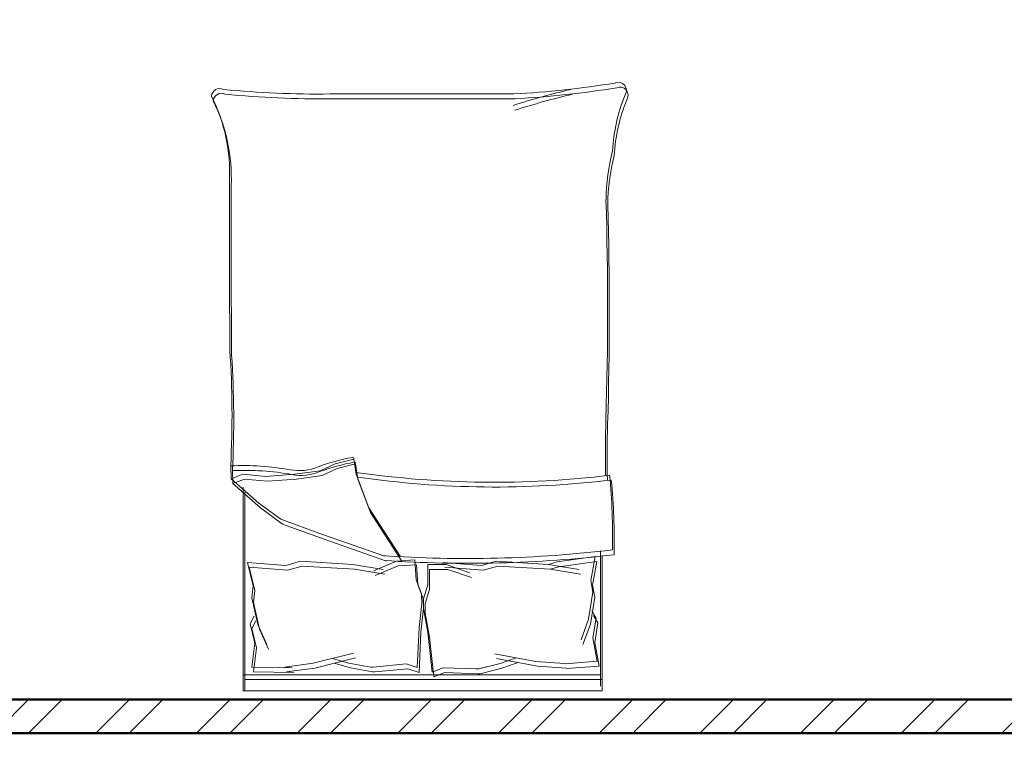
# Model space of a CAD drawing. Units: inches. Extents: x 963 to 2075, y 289 to 2657.
# Tile 15 of 98: x 1179 to 1310, y 1818 to 1917. Entities that reach past the tile are written whole.
import ezdxf

# ---------------------------------------------------------------- set-up
doc = ezdxf.new("R2010")
doc.units = ezdxf.units.IN
for name, color, linetype, lineweight in [('A-FURN', 8, 'Continuous', 18), ('A-WALL', 7, 'Continuous', 50), ('A-WALL-PATT', 8, 'Continuous', 13)]:
    doc.layers.add(name, color=color, linetype=linetype, lineweight=lineweight)

# ---------------------------------------------------------------- blocks, each defined once
blk = doc.blocks.new('BED-DOUBLE')
for p, q in [((1236.12, 2450.52), (1254.23, 2450.52)), ((1236.12, 2450.52), (1254.23, 2450.52)), ((1236.76, 2450.75), (1254.87, 2450.75)), ((1236.76, 2450.75), (1254.87, 2450.75)), ((1251.56, 2450.33), (1248.37, 2449.75)), ((1251.56, 2450.33), (1248.37, 2449.75)), ((1251.53, 2450.32), (1251.86, 2446.04)), ((1251.53, 2450.32), (1251.86, 2446.04)), ((1252.7, 2450.52), (1252.7, 2402.73)), ((1252.7, 2450.52), (1252.7, 2402.73)), ((1253.34, 2450.75), (1253.34, 2402.96)), ((1253.34, 2450.75), (1253.34, 2402.96)), ((1254.87, 2450.75), (1254.87, 2402.73)), ((1237.61, 2444.71), (1236.89, 2449.81)), ((1236.89, 2449.81), (1240.07, 2449.23)), ((1237.61, 2444.71), (1236.89, 2449.81)), ((1236.89, 2449.81), (1240.07, 2449.23)), ((1238.25, 2444.94), (1237.53, 2450.04)), ((1237.53, 2450.04), (1240.71, 2449.46)), ((1238.25, 2444.94), (1237.53, 2450.04)), ((1237.53, 2450.04), (1240.71, 2449.46)), ((1240.07, 2449.23), (1241.66, 2449.52)), ((1240.07, 2449.23), (1241.66, 2449.52)), ((1240.71, 2449.46), (1242.3, 2449.75)), ((1240.71, 2449.46), (1242.3, 2449.75)), ((1241.66, 2449.52), (1245.28, 2448.94)), ((1241.66, 2449.52), (1245.28, 2448.94)), ((1242.3, 2449.75), (1245.92, 2449.17)), ((1242.3, 2449.75), (1245.92, 2449.17)), ((1245.13, 2449.96), (1244.12, 2449.38)), ((1245.13, 2449.96), (1244.12, 2449.38)), ((1245.77, 2450.18), (1244.76, 2449.61)), ((1245.77, 2450.18), (1244.76, 2449.61)), ((1247.74, 2449.52), (1245.13, 2449.96)), ((1247.74, 2449.52), (1245.13, 2449.96)), ((1245.28, 2448.94), (1248.02, 2447.93)), ((1245.28, 2448.94), (1248.02, 2447.93)), ((1248.37, 2449.75), (1245.77, 2450.18)), ((1248.37, 2449.75), (1245.77, 2450.18)), ((1245.92, 2449.17), (1248.66, 2448.16)), ((1245.92, 2449.17), (1248.66, 2448.16)), ((1250.92, 2450.1), (1247.74, 2449.52)), ((1250.92, 2450.1), (1247.74, 2449.52)), ((1250.89, 2450.1), (1251.22, 2445.82)), ((1250.89, 2450.1), (1251.22, 2445.82)), ((1238.6, 2447.61), (1237.94, 2443.58)), ((1238.6, 2447.61), (1237.94, 2443.58)), ((1239.24, 2447.84), (1238.58, 2443.81)), ((1239.24, 2447.84), (1238.58, 2443.81)), ((1251.21, 2445.71), (1250.92, 2441.89)), ((1251.21, 2445.71), (1250.92, 2441.89)), ((1251.22, 2445.82), (1251.21, 2445.71)), ((1251.22, 2445.82), (1251.21, 2445.71)), ((1251.84, 2445.94), (1251.56, 2442.11)), ((1251.84, 2445.94), (1251.56, 2442.11)), ((1251.86, 2446.04), (1251.84, 2445.94)), ((1251.86, 2446.04), (1251.84, 2445.94)), ((1237.94, 2443.58), (1237.61, 2444.71)), ((1237.94, 2443.58), (1237.61, 2444.71)), ((1238.58, 2443.81), (1238.15, 2436.8)), ((1238.58, 2443.81), (1238.15, 2436.8)), ((1238.58, 2443.81), (1238.25, 2444.94)), ((1238.58, 2443.81), (1238.25, 2444.94)), ((1237.94, 2443.58), (1237.51, 2436.57)), ((1237.94, 2443.58), (1237.51, 2436.57)), ((1250.92, 2441.89), (1249.9, 2436.39)), ((1250.92, 2441.89), (1249.9, 2436.39)), ((1251.56, 2442.11), (1250.54, 2436.62)), ((1251.56, 2442.11), (1250.54, 2436.62)), ((1174.99, 2438.93), (1174.99, 2414.32)), ((1174.99, 2438.93), (1174.99, 2414.32)), ((1175.63, 2439.16), (1175.63, 2414.55)), ((1175.63, 2439.16), (1175.63, 2414.55)), ((1250.48, 2439.14), (1251.21, 2437.12)), ((1250.48, 2439.14), (1251.21, 2437.12)), ((1251.12, 2439.37), (1251.84, 2437.34)), ((1251.12, 2439.37), (1251.84, 2437.34)), ((1251.21, 2437.12), (1251.93, 2434.22)), ((1251.21, 2437.12), (1251.93, 2434.23)), ((1251.84, 2437.34), (1252.57, 2434.45)), ((1251.84, 2437.34), (1252.57, 2434.45)), ((1237.51, 2436.57), (1238.06, 2434.61)), ((1237.51, 2436.57), (1238.06, 2434.61)), ((1238.15, 2436.8), (1238.7, 2434.84)), ((1238.15, 2436.8), (1238.7, 2434.84)), ((1238.06, 2434.61), (1237.66, 2429.48)), ((1238.06, 2434.61), (1237.66, 2429.48)), ((1238.7, 2434.84), (1238.3, 2429.71)), ((1238.7, 2434.84), (1238.3, 2429.71)), ((1252.57, 2434.45), (1252.57, 2434.13)), ((1252.57, 2434.45), (1252.57, 2434.13)), ((1238.61, 2430.12), (1239.7, 2433.26)), ((1238.61, 2430.12), (1239.7, 2433.26)), ((1251.93, 2433.9), (1251.78, 2429.46)), ((1251.93, 2433.9), (1251.78, 2429.46)), ((1251.93, 2434.23), (1251.93, 2433.9)), ((1251.93, 2434.22), (1251.93, 2433.9)), ((1252.57, 2434.13), (1252.42, 2429.69)), ((1252.57, 2434.13), (1252.42, 2429.69)), ((1237.97, 2429.89), (1239.06, 2433.04)), ((1237.97, 2429.89), (1239.06, 2433.04)), ((1237.97, 2427.43), (1237.97, 2429.89)), ((1237.97, 2427.43), (1237.97, 2429.89)), ((1238.61, 2427.66), (1238.61, 2430.12)), ((1238.61, 2427.66), (1238.61, 2430.12)), ((1251.78, 2429.46), (1252.36, 2428.01)), ((1251.78, 2429.46), (1252.36, 2428.01)), ((1252.42, 2429.69), (1253, 2428.24)), ((1252.42, 2429.69), (1253, 2428.24)), ((1252.36, 2428.01), (1247.01, 2427.43)), ((1252.36, 2428.01), (1247.01, 2427.43)), ((1253, 2428.24), (1247.65, 2427.66)), ((1253, 2428.24), (1247.65, 2427.66)), ((1240.65, 2427.43), (1237.97, 2427.43)), ((1240.65, 2427.43), (1237.97, 2427.43)), ((1241.29, 2427.66), (1238.61, 2427.66)), ((1241.29, 2427.66), (1238.61, 2427.66)), ((1241.86, 2426.56), (1240.02, 2425.86)), ((1241.86, 2426.56), (1240.02, 2425.86)), ((1242.53, 2426.86), (1240.65, 2427.43)), ((1242.53, 2426.86), (1240.65, 2427.43)), ((1242.49, 2426.79), (1240.66, 2426.09)), ((1242.49, 2426.79), (1240.66, 2426.09)), ((1243.17, 2427.08), (1241.29, 2427.66)), ((1243.17, 2427.08), (1241.29, 2427.66)), ((1243.15, 2426.64), (1241.86, 2426.56)), ((1243.15, 2426.64), (1241.86, 2426.56)), ((1243.79, 2426.87), (1242.49, 2426.79)), ((1243.79, 2426.87), (1242.49, 2426.79)), ((1243.83, 2426.86), (1242.53, 2426.86)), ((1243.83, 2426.86), (1242.53, 2426.86)), ((1246.37, 2426.26), (1243.15, 2426.64)), ((1246.37, 2426.26), (1243.15, 2426.64)), ((1244.47, 2427.08), (1243.17, 2427.08)), ((1244.47, 2427.08), (1243.17, 2427.08)), ((1247, 2426.49), (1243.79, 2426.87)), ((1247, 2426.49), (1243.79, 2426.87)), ((1247.01, 2427.43), (1243.83, 2426.86)), ((1247.01, 2427.43), (1243.83, 2426.86)), ((1247.65, 2427.66), (1244.47, 2427.08)), ((1247.65, 2427.66), (1244.47, 2427.08)), ((1240.02, 2425.86), (1237.34, 2425.7)), ((1240.02, 2425.86), (1237.34, 2425.7)), ((1237.34, 2425.7), (1237.49, 2423.24)), ((1237.34, 2425.7), (1237.49, 2423.24)), ((1240.66, 2426.09), (1237.98, 2425.93)), ((1240.66, 2426.09), (1237.98, 2425.93)), ((1237.98, 2425.93), (1238.13, 2423.47)), ((1237.98, 2425.93), (1238.13, 2423.47)), ((1251.74, 2426.02), (1246.37, 2426.26)), ((1251.74, 2426.02), (1246.37, 2426.26)), ((1252.38, 2426.25), (1247, 2426.49)), ((1252.38, 2426.25), (1247, 2426.49)), ((1251.25, 2424.54), (1251.74, 2426.02)), ((1251.25, 2424.54), (1251.74, 2426.02)), ((1251.89, 2424.77), (1252.38, 2426.25)), ((1251.89, 2424.77), (1252.38, 2426.25)), ((1237.49, 2423.96), (1231, 2419.77)), ((1237.49, 2423.96), (1231, 2419.77)), ((1251.68, 2420.11), (1251.25, 2424.54)), ((1251.68, 2420.11), (1251.25, 2424.54)), ((1252.31, 2420.34), (1251.89, 2424.77)), ((1252.31, 2420.34), (1251.89, 2424.77)), ((1236.85, 2423.74), (1230.36, 2419.55)), ((1236.85, 2423.74), (1230.36, 2419.55)), ((1237.49, 2423.24), (1238.78, 2420.17)), ((1237.49, 2423.24), (1238.78, 2420.17)), ((1238.13, 2423.47), (1239.42, 2420.4)), ((1238.13, 2423.47), (1239.42, 2420.4)), ((1233.92, 2413.35), (1236.85, 2421.69)), ((1233.92, 2413.35), (1236.85, 2421.69)), ((1234.56, 2413.58), (1237.49, 2421.92)), ((1234.56, 2413.58), (1237.49, 2421.92)), ((1238.6, 2421.43), (1237.94, 2417.4)), ((1238.6, 2421.43), (1237.94, 2417.4)), ((1239.24, 2421.66), (1238.58, 2417.63)), ((1239.24, 2421.66), (1238.58, 2417.63)), ((1251.7, 2419.79), (1251.68, 2420.11)), ((1251.7, 2419.79), (1251.68, 2420.11)), ((1251.79, 2417.09), (1252.33, 2420.02)), ((1251.79, 2417.09), (1252.33, 2420.02)), ((1252.33, 2420.02), (1252.31, 2420.34)), ((1252.33, 2420.02), (1252.31, 2420.34)), ((1230.36, 2419.55), (1225.87, 2417.84)), ((1230.36, 2419.55), (1225.87, 2417.84)), ((1231, 2419.77), (1226.51, 2418.07)), ((1231, 2419.77), (1226.51, 2418.07)), ((1251.15, 2416.86), (1251.7, 2419.79)), ((1251.15, 2416.86), (1251.7, 2419.79)), ((1225.87, 2417.84), (1223.86, 2417.53)), ((1225.87, 2417.84), (1223.86, 2417.53)), ((1223.86, 2417.53), (1224.47, 2415.05)), ((1223.86, 2417.53), (1224.47, 2415.05)), ((1226.51, 2418.07), (1224.49, 2417.76)), ((1226.51, 2418.07), (1224.49, 2417.76)), ((1224.49, 2417.76), (1225.11, 2415.28)), ((1224.49, 2417.76), (1225.11, 2415.28)), ((1237.94, 2417.4), (1237.51, 2410.39)), ((1237.94, 2417.4), (1237.51, 2410.39)), ((1238.58, 2417.63), (1238.15, 2410.62)), ((1238.58, 2417.63), (1238.15, 2410.62)), ((1251.16, 2412.08), (1249.81, 2417.5)), ((1251.16, 2412.08), (1249.81, 2417.5)), ((1251.8, 2412.31), (1250.45, 2417.73)), ((1251.8, 2412.31), (1250.45, 2417.73)), ((1250.56, 2414.79), (1251.15, 2416.86)), ((1250.56, 2414.79), (1251.15, 2416.86)), ((1251.2, 2415.02), (1251.79, 2417.09)), ((1251.2, 2415.02), (1251.79, 2417.09)), ((1224.47, 2415.05), (1225.4, 2413.04)), ((1224.47, 2415.05), (1225.4, 2413.04)), ((1225.11, 2415.28), (1226.04, 2413.27)), ((1225.11, 2415.28), (1226.04, 2413.27)), ((1231.9, 2407.77), (1233.92, 2413.35)), ((1231.9, 2407.78), (1233.92, 2413.35)), ((1232.54, 2408), (1234.56, 2413.58)), ((1232.54, 2408), (1234.56, 2413.58)), ((1225.4, 2413.04), (1225.87, 2409.63)), ((1225.4, 2413.04), (1225.87, 2409.63)), ((1226.04, 2413.27), (1226.51, 2409.86)), ((1226.04, 2413.27), (1226.51, 2409.86)), ((1251.69, 2408.28), (1251.16, 2412.08)), ((1251.69, 2408.28), (1251.16, 2412.08)), ((1252.33, 2408.51), (1251.8, 2412.31)), ((1252.33, 2408.51), (1251.8, 2412.31)), ((1225.87, 2409.63), (1226.18, 2405.76)), ((1225.87, 2409.63), (1226.18, 2405.76)), ((1226.51, 2409.86), (1226.82, 2405.99)), ((1226.51, 2409.86), (1226.82, 2405.99)), ((1237.51, 2410.39), (1238.06, 2408.43)), ((1237.51, 2410.39), (1238.06, 2408.43)), ((1238.15, 2410.62), (1238.7, 2408.66)), ((1238.15, 2410.62), (1238.7, 2408.66)), ((1252.31, 2404.11), (1252.41, 2409.51)), ((1252.31, 2404.11), (1252.41, 2409.51)), ((1252.41, 2409.51), (1252.33, 2408.51)), ((1252.41, 2409.51), (1252.33, 2408.51)), ((1238.06, 2408.43), (1237.66, 2403.3)), ((1238.06, 2408.43), (1237.66, 2403.3)), ((1238.7, 2408.66), (1238.3, 2403.52)), ((1238.7, 2408.66), (1238.3, 2403.52)), ((1251.68, 2403.88), (1251.77, 2409.29)), ((1251.68, 2403.88), (1251.77, 2409.28)), ((1251.77, 2409.29), (1251.69, 2408.28)), ((1251.77, 2409.28), (1251.69, 2408.28)), ((1229.74, 2404.83), (1231.9, 2407.78)), ((1229.74, 2404.83), (1231.9, 2407.77)), ((1230.38, 2405.06), (1232.54, 2408)), ((1230.38, 2405.06), (1232.54, 2408)), ((1226.18, 2405.76), (1225.87, 2402.66)), ((1226.18, 2405.76), (1225.87, 2402.66)), ((1226.82, 2405.99), (1226.51, 2402.89)), ((1226.82, 2405.99), (1226.51, 2402.89)), ((1245.98, 2404.69), (1248.65, 2405.87)), ((1245.98, 2404.69), (1248.65, 2405.87)), ((1246.61, 2404.91), (1249.29, 2406.1)), ((1246.61, 2404.91), (1249.29, 2406.09)), ((1226.49, 2401.13), (1229.74, 2404.83)), ((1226.49, 2401.13), (1229.74, 2404.83)), ((1227.13, 2401.36), (1230.38, 2405.06)), ((1227.13, 2401.36), (1230.38, 2405.06)), ((1238.3, 2403.52), (1241.44, 2404.3)), ((1238.3, 2403.52), (1241.44, 2404.3)), ((1241.44, 2404.3), (1243.04, 2404.11)), ((1241.44, 2404.3), (1243.04, 2404.11)), ((1242.4, 2403.88), (1245.98, 2404.69)), ((1242.4, 2403.88), (1245.98, 2404.69)), ((1243.04, 2404.11), (1246.61, 2404.91)), ((1243.04, 2404.11), (1246.61, 2404.91)), ((1245.89, 2403.67), (1244.85, 2404.18)), ((1245.89, 2403.67), (1244.85, 2404.18)), ((1246.53, 2403.89), (1245.49, 2404.41)), ((1246.53, 2403.89), (1245.49, 2404.41)), ((1248.46, 2404.26), (1245.89, 2403.67)), ((1248.46, 2404.26), (1245.89, 2403.67)), ((1249.1, 2404.49), (1246.53, 2403.89)), ((1249.1, 2404.49), (1246.53, 2403.89)), ((1251.68, 2403.88), (1248.46, 2404.26)), ((1251.68, 2403.88), (1248.46, 2404.26)), ((1252.31, 2404.11), (1249.1, 2404.49)), ((1252.31, 2404.11), (1249.1, 2404.49)), ((1226.51, 2402.89), (1227.13, 2401.36)), ((1226.51, 2402.89), (1227.13, 2401.36)), ((1254.87, 2402.96), (1228.26, 2402.96)), ((1254.87, 2402.96), (1228.26, 2402.96)), ((1237.66, 2403.3), (1240.8, 2404.07)), ((1237.66, 2403.3), (1240.8, 2404.07)), ((1240.8, 2404.07), (1242.4, 2403.88)), ((1240.8, 2404.07), (1242.4, 2403.88)), ((1225.87, 2402.66), (1226.49, 2401.13)), ((1225.87, 2402.66), (1226.49, 2401.13)), ((1254.23, 2402.73), (1227.62, 2402.73)), ((1254.23, 2402.73), (1227.62, 2402.73)), ((1254.87, 2402.73), (1254.23, 2402.73)), ((1224.74, 2401.05), (1226.49, 2401.13, 3.87)), ((1224.74, 2401.05), (1226.49, 2401.13, 3.87)), ((1225.38, 2401.28), (1227.13, 2401.36, 3.87)), ((1225.38, 2401.28), (1227.13, 2401.36, 3.87))]:
    blk.add_line(p, q)
for centre, radius, start, end in [((1175.15, 2453.14), 1.09, 56.1736, 203.4781), ((1175.15, 2453.14), 1.09, 56.1736, 203.4781), ((1174.51, 2452.91), 1.09, 56.1736, 203.4781), ((1174.51, 2452.91), 1.09, 56.1736, 203.4781), ((1183.96, 2475.65), 23.56, 247.9751, 266.652), ((1183.96, 2475.65), 23.56, 247.9751, 266.652), ((1184.6, 2475.88), 23.56, 247.9751, 266.652), ((1184.6, 2475.88), 23.56, 247.9751, 266.652), ((1053.4, 2432.57), 121.76, 2.9958, 9.4091), ((1053.4, 2432.57), 121.76, 2.9958, 9.4091), ((1054.03, 2432.8), 121.76, 2.9958, 9.4091), ((1054.03, 2432.8), 121.76, 2.9958, 9.4091), ((1189.72, 2480.89), 29.63, 256.0648, 268.9113), ((1189.72, 2480.89), 29.63, 256.0648, 268.9113), ((1190.36, 2481.12), 29.63, 256.0648, 268.9113), ((1190.36, 2481.12), 29.63, 256.0648, 268.9113), ((1204.26, 1969.4), 482.31, 88.2277, 91.7185), ((1204.26, 1969.4), 482.31, 88.2277, 91.7185), ((1097.92, 2436.24), 129.02, 351.7845, 6.9006), ((1097.92, 2436.24), 129.02, 351.7845, 6.9006), ((1234.14, 2368.83), 83.31, 88.7218, 95.604), ((1234.14, 2368.83), 83.31, 88.7218, 95.604), ((1098.56, 2436.47), 129.02, 351.7845, 6.9006), ((1098.56, 2436.47), 129.02, 351.7845, 6.9006), ((1234.78, 2369.06), 83.31, 88.7218, 95.604), ((1234.78, 2369.06), 83.31, 88.7218, 95.604), ((1072.18, 2432.64), 164.97, 356.0865, 6.7821), ((1072.18, 2432.64), 164.97, 356.0865, 6.7821), ((1072.82, 2432.86), 164.97, 356.0865, 6.7821), ((1072.82, 2432.86), 164.97, 356.0865, 6.7821), ((1203.62, 1969.17), 482.31, 88.2277, 91.7185), ((1203.62, 1969.17), 482.31, 88.2277, 91.7185), ((1223.06, 2621.3), 170.11, 268.4762, 271.0082), ((1223.06, 2621.3), 170.11, 268.4762, 271.0082), ((1223.7, 2621.53), 170.11, 268.4762, 271.0082), ((1223.7, 2621.53), 170.11, 268.4762, 271.0082), ((1277.94, 2471.22), 106.46, 193.3832, 197.7053), ((1277.94, 2471.22), 106.46, 193.3832, 197.7053), ((1278.58, 2471.44), 106.46, 193.3832, 197.7053), ((1278.58, 2471.44), 106.46, 193.3832, 197.7053), ((1223.79, 2417.36), 0.185, 70.2464, 181.1377), ((1223.79, 2417.36), 0.185, 70.2464, 181.1377), ((1252.75, 2422.84), 29.65, 190.6617, 199.8806), ((1252.75, 2422.84), 29.65, 190.6617, 199.8806), ((1224.43, 2417.59), 0.185, 70.2464, 181.1377), ((1224.43, 2417.59), 0.185, 70.2464, 181.1377), ((1253.39, 2423.07), 29.65, 190.6617, 199.8806), ((1253.39, 2423.07), 29.65, 190.6617, 199.8806), ((1041.96, 2412.84), 133.04, 354.4998, 0.6351), ((1041.96, 2412.84), 133.04, 354.4998, 0.6351), ((1042.6, 2413.07), 133.04, 354.4998, 0.6351), ((1042.6, 2413.07), 133.04, 354.4998, 0.6351), ((1219.17, 2410.25), 6.22, 348.6608, 23.7384), ((1219.17, 2410.25), 6.22, 348.6608, 23.7384), ((1219.81, 2410.48), 6.22, 348.6608, 23.7384), ((1219.81, 2410.48), 6.22, 348.6608, 23.7384), ((1260.89, 2402.67), 36.18, 169.8763, 182.5657), ((1260.89, 2402.67), 36.18, 169.8763, 182.5657), ((1261.53, 2402.9), 36.18, 169.8763, 182.5657), ((1261.53, 2402.9), 36.18, 169.8763, 182.5657), ((1176, 2399.81), 1.1, 152.6588, 266.02), ((1176, 2399.81), 1.1, 152.6588, 266.02), ((1185.57, 2377.84), 23.07, 87.4714, 116.4681), ((1185.57, 2377.84), 23.07, 87.4714, 116.4681), ((1186.21, 2378.07), 23.07, 87.4714, 116.4681), ((1186.21, 2378.07), 23.07, 87.4714, 116.4681), ((1186.41, 6962.74), 4561.86, 270.00217, 270.28689), ((1186.41, 6962.74), 4561.86, 270.00217, 270.28689), ((1187.05, 6962.97), 4561.86, 270.00217, 270.28689), ((1187.05, 6962.97), 4561.86, 270.00217, 270.28689), ((1217.92, 2271.73), 129.5, 86.9791, 93.8365), ((1217.92, 2271.73), 129.5, 86.9791, 93.8365), ((1218.56, 2271.96), 129.5, 86.9791, 93.8365), ((1218.56, 2271.96), 129.5, 86.9791, 93.8365), ((1175.36, 2399.58), 1.1, 152.6588, 266.02), ((1175.36, 2399.58), 1.1, 152.6588, 266.02)]:
    blk.add_arc(centre, radius, start, end)

msp = doc.modelspace()

# ---------------------------------------------------------------- hatches: boundary and pattern name
at = {"layer": 'A-WALL-PATT'}
h = msp.add_hatch(dxfattribs=at)
h.set_pattern_fill('ANSI32', color=256)
h.paths.add_polyline_path([(1473.61, 2163.07), (1473.61, 2165.32), (1376.42, 2165.32), (1376.42, 2227.98), (1371.92, 2227.98), (1371.92, 2214.82), (1368.41, 2214.82), (1368.41, 2210.32), (1371.92, 2210.32), (1371.92, 2160.82), (1395.92, 2160.82), (1395.92, 2090.32), (1217.34, 2090.32), (1217.34, 2085.82), (1395.92, 2085.82), (1458.92, 2085.82), (1458.92, 2108.32), (1454.42, 2108.32), (1454.42, 2090.32), (1400.42, 2090.32), (1400.42, 2160.82), (1473.61, 2160.82)])
h.paths.add_polyline_path([(1649.42, 2210.32), (1653.23, 2210.32), (1653.23, 2214.82), (1649.42, 2214.82), (1649.42, 2227.98), (1644.92, 2227.98), (1644.92, 2165.32), (1550.1, 2165.32), (1550.1, 2160.82), (1620.92, 2160.82), (1620.92, 2112.82), (1555.45, 2112.82), (1555.45, 2108.32), (1584.33, 2108.32), (1584.33, 2084.92), (1588.83, 2084.92), (1588.83, 2108.32), (1625.42, 2108.32), (1667.95, 2108.32), (1667.95, 2022.67), (1588.83, 2022.67), (1588.83, 2047.41), (1584.33, 2047.41), (1584.33, 1996), (1588.83, 1996), (1588.83, 2018.32), (1667.95, 2018.17), (1667.95, 1928.32), (1625.42, 1928.32), (1625.42, 1923.82), (1672.45, 1923.82), (1672.45, 1928.32), (1672.45, 1946.66), (1785.45, 1946.66), (1785.45, 1951.16), (1743.03, 1951.16), (1743.03, 2017.92), (1841.42, 2017.92), (1841.42, 2014.77), (1845.92, 2014.77), (1845.92, 2017.92), (1905.92, 2017.92), (1905.92, 1987.51), (1910.42, 1987.51), (1910.42, 2022.42), (1910.42, 2068.52), (1905.92, 2068.52), (1905.92, 2022.42), (1845.92, 2022.42), (1845.92, 2025.85), (1843.67, 2025.85), (1841.42, 2025.85), (1841.42, 2022.42), (1743.03, 2022.42), (1743.03, 2084.03), (1768.45, 2084.03), (1785.45, 2084.03), (1785.45, 2088.53), (1672.45, 2088.53), (1672.45, 2112.82), (1667.95, 2112.82), (1625.42, 2112.82), (1625.42, 2160.82), (1649.42, 2160.82)])
h.paths.add_polyline_path([(1672.45, 2084.03), (1738.53, 2084.03), (1738.53, 1951.16), (1672.45, 1951.16)], flags=16)
h.paths.add_polyline_path([(1672.45, 2084.03), (1738.53, 2084.03), (1705.49, 2017.6)], flags=0)
h.paths.add_polyline_path([(1262.77, 2085.82), (1258.27, 2085.82), (1258.27, 2023.28), (1184.42, 2023.28), (1184.42, 2018.78), (1258.27, 2018.78), (1258.27, 1950.82), (1262.77, 1950.82)])
h.paths.add_polyline_path([(1312.27, 2085.82), (1307.77, 2085.82), (1307.77, 1950.82), (1312.27, 1950.82)])
h.paths.add_polyline_path([(1458.92, 1950.82), (1395.92, 1950.82), (1216.57, 1950.82), (1216.57, 1946.32), (1346.42, 1946.32), (1395.92, 1946.32), (1395.92, 1875.82), (1371.92, 1875.82), (1371.92, 1826.32), (1368.93, 1826.32), (1368.93, 1821.82), (1371.92, 1821.82), (1371.92, 1813.62), (1376.42, 1813.62), (1376.42, 1871.32), (1474.5, 1871.32), (1474.5, 1873.57), (1474.5, 1875.82), (1400.42, 1875.82), (1400.42, 1946.32), (1454.42, 1946.32), (1454.42, 1928.32), (1458.92, 1928.32)])
h.paths.add_polyline_path([(1184.42, 2120.78), (1167.92, 2120.78), (1167.92, 2134.81), (1165.67, 2134.81), (1163.42, 2134.81), (1163.42, 2120.78), (1119.92, 2120.78), (1119.92, 2098.1), (1124.42, 2098.1), (1124.42, 2116.28), (1167.92, 2116.28), (1179.92, 2116.28), (1179.92, 2045.92), (1184.42, 2045.92), (1184.42, 2090.32), (1184.42, 2116.28)])
h.paths.add_polyline_path([(1124.42, 2018.78), (1179.92, 2018.78), (1179.92, 2016.29), (1184.42, 2016.29), (1184.42, 2023.28), (1184.42, 2026.59), (1182.17, 2026.59), (1179.92, 2026.59), (1179.92, 2023.28), (1124.42, 2023.28), (1124.42, 2074.1), (1119.92, 2074.1), (1119.92, 2018.78), (1119.92, 1979.63), (1124.42, 1979.63)])
h.paths.add_polyline_path([(1184.42, 1925.78), (1184.42, 1946.32), (1184.42, 1996.07), (1182.17, 1996.07), (1179.92, 1996.07), (1179.92, 1925.78), (1124.42, 1925.78), (1124.42, 1955.63), (1119.92, 1955.5), (1119.92, 1921.28), (1158.92, 1921.28), (1158.92, 1909.98), (1163.42, 1909.98), (1163.42, 1921.28), (1184.42, 1921.28)])
h.paths.add_polyline_path([(1341.45, 1826.32), (1163.42, 1826.32), (1163.42, 1849.98), (1158.92, 1849.98), (1158.92, 1821.82), (1158.92, 1804.03), (1163.42, 1804.03), (1163.42, 1821.82), (1341.45, 1821.82)])
h.paths.add_polyline_path([(1222.98, 1713.82), (1163.42, 1713.82), (1163.42, 1744.03), (1161.17, 1744.03), (1158.92, 1744.03), (1158.92, 1713.82), (1119.92, 1713.82), (1119.92, 1694.65), (1124.42, 1694.65), (1124.42, 1709.32), (1158.92, 1709.32), (1222.98, 1709.32)])
h.paths.add_polyline_path([(1328.42, 1713.82), (1252.04, 1713.82), (1252.04, 1711.57), (1252.04, 1709.32), (1256.42, 1709.32), (1256.42, 1547.32), (1232.94, 1547.32), (1232.94, 1545.07), (1232.94, 1542.82), (1292.42, 1542.82), (1292.42, 1527.63), (1296.92, 1527.63), (1296.92, 1542.82), (1299.46, 1542.82), (1299.46, 1547.32), (1260.92, 1547.32), (1260.92, 1658.32), (1343.66, 1658.32), (1343.66, 1660.57), (1343.66, 1662.82), (1328.42, 1662.82), (1328.42, 1676.59), (1327.4, 1676.59), (1323.92, 1676.59), (1323.92, 1662.82), (1260.92, 1662.82), (1260.92, 1709.32), (1323.92, 1709.32), (1323.92, 1699.85), (1328.42, 1699.85)])
h.paths.add_polyline_path([(1649.42, 1875.82), (1625.42, 1875.82), (1625.42, 1928.32), (1620.92, 1928.32), (1588.83, 1928.32), (1588.83, 1950.59), (1584.33, 1950.59), (1584.33, 1928.32), (1555.45, 1928.32), (1555.45, 1923.82), (1620.92, 1923.82), (1620.92, 1875.82), (1548.95, 1875.82), (1548.95, 1873.57), (1548.95, 1871.32), (1644.92, 1871.32), (1644.92, 1813.62), (1649.42, 1813.62), (1649.42, 1821.82), (1652.04, 1821.82), (1652.04, 1824.07), (1652.04, 1826.32), (1649.42, 1826.32)])
h.paths.add_polyline_path([(1512.92, 1871.32), (1516.48, 1871.32), (1516.48, 1875.82), (1512.92, 1875.82), (1512.92, 1923.82), (1512.92, 1928.32), (1512.92, 1930.83), (1508.42, 1930.83), (1508.42, 1875.82), (1504.41, 1875.82), (1504.41, 1871.32), (1508.42, 1871.32), (1508.42, 1713.82), (1376.42, 1713.82), (1376.42, 1743.32), (1371.92, 1743.32), (1371.92, 1709.32), (1371.92, 1706.01), (1376.42, 1706.01), (1376.42, 1709.32), (1508.42, 1709.32), (1508.42, 1547.32), (1501.87, 1547.32), (1501.87, 1542.82), (1508.42, 1542.82), (1508.42, 1482.82), (1508.42, 1436.32), (1512.92, 1436.32), (1512.92, 1542.82), (1519.32, 1542.82), (1519.32, 1545.07), (1519.32, 1547.32), (1512.92, 1547.32), (1512.92, 1709.32), (1644.92, 1709.32), (1644.92, 1707.55), (1649.42, 1707.55), (1649.42, 1709.32), (1649.42, 1743.32), (1644.92, 1743.32), (1644.92, 1713.82), (1512.92, 1713.82)])
h.paths.add_polyline_path([(1129.88, 1545.07), (1129.88, 1547.32), (1124.42, 1547.32), (1095.92, 1547.32), (1095.92, 1614.82), (1124.42, 1614.82), (1124.42, 1619.32), (1095.92, 1619.32), (1091.42, 1619.32), (1091.42, 1542.82), (1095.92, 1542.82), (1119.92, 1542.82), (1129.88, 1542.82)])
h.paths.add_polyline_path([(1208.42, 1542.82), (1211.74, 1542.82), (1211.74, 1547.32), (1198.85, 1547.32), (1198.85, 1542.82), (1203.92, 1542.82), (1203.92, 1478.32), (1208.42, 1478.32), (1296.92, 1478.32), (1296.92, 1503.63), (1292.42, 1503.63), (1292.42, 1482.82), (1208.42, 1482.82)])
h.paths.add_polyline_path([(1430.42, 1542.82), (1435.7, 1542.82), (1435.7, 1545.07), (1435.7, 1547.32), (1422.66, 1547.32), (1422.66, 1545.07), (1422.66, 1542.82), (1425.92, 1542.82), (1425.92, 1482.86), (1341.92, 1482.86), (1341.92, 1502.73), (1337.42, 1502.73), (1337.42, 1478.36), (1425.92, 1478.36), (1425.92, 1440.82), (1425.92, 1436.32), (1430.42, 1436.32)])
h.paths.add_polyline_path([(1698.48, 2004.26), (1727.69, 2004.26), (1727.69, 2022.92), (1698.48, 2022.92)], flags=8)

# ---------------------------------------------------------------- linework, layer by layer
at = {"layer": 'A-WALL'}
for p, q in [((1163.42, 1826.32), (1342.58, 1826.32)), ((1341.45, 1821.82), (1163.42, 1821.82))]:
    msp.add_line(p, q, dxfattribs=at)

# ---------------------------------------------------------------- block references
at = {"layer": 'A-FURN', "rotation": 269.9999998331857}
msp.add_blockref('BED-DOUBLE', (-1194.28, 3082.34), dxfattribs=at)

doc.saveas('drawing.dxf')
